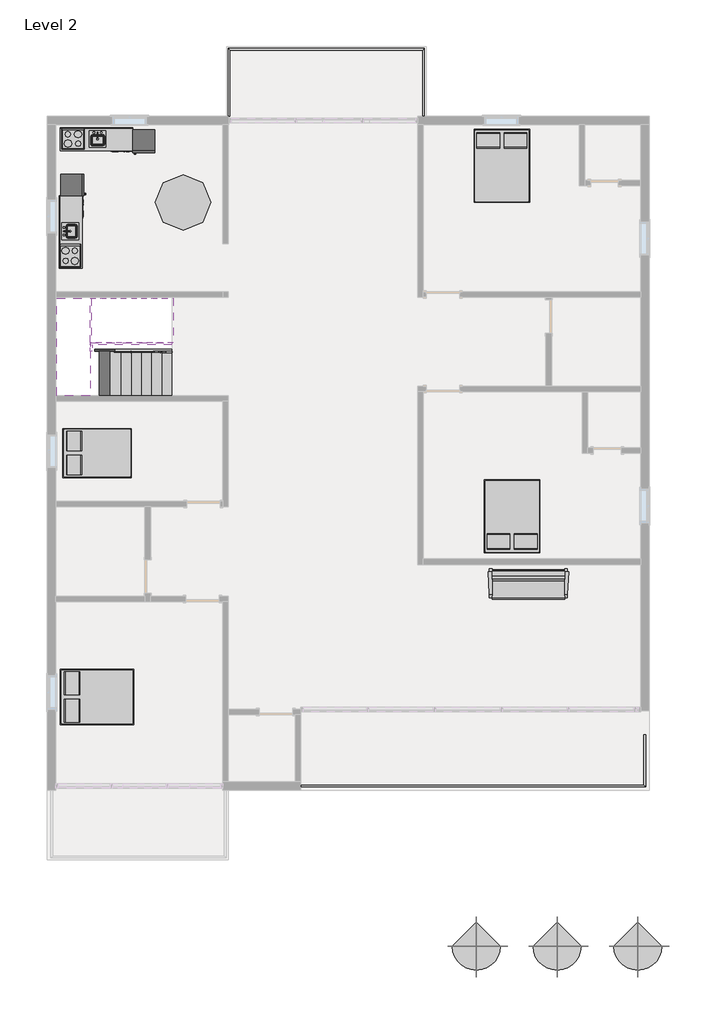
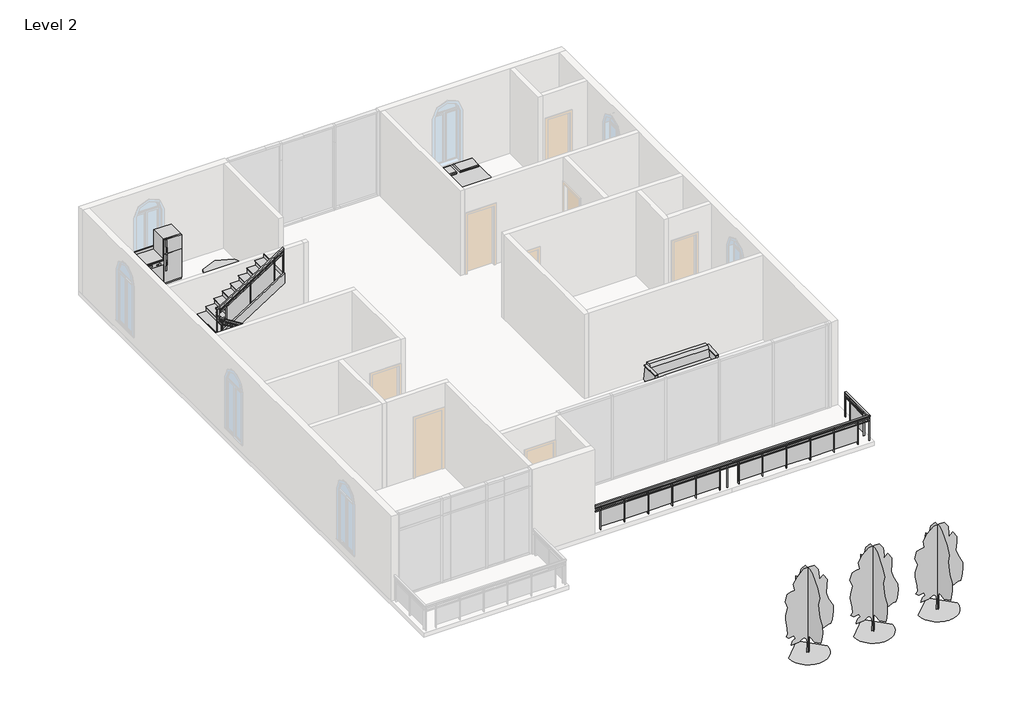
# One storey, part 3 of 3: 8 furniture elements, 8 proxies, 3 geographic elements, 3 members, 3 railings, 2 flow terminals, 2 stair flights, 1 slab.
"""IFC4 building model written with IfcOpenShell, lengths in millimetres."""

from ifc_helpers import new_model, si_unit, frame, origin, place, context, project, spatial, polyline, outline, extrude, faceted_brep, transform, mapped, element, save
from components import proxy_a6faaae8, proxy_45b28599, kitchenette_medium_kitchenette_medium_844211aa, proxy_c523a7b7, flow_terminal_871c2e40, furniture_c8abb964, furniture_1d2926bd, furniture_c6510c7c, furniture_aff9b2fb, furniture_bbcc68ce, rpc_tree_deciduous_red_ash_25_5dd3353f, non_monolithic_landing_6f104080, stair_flight_d31f5684, stair_flight_e2acd8df

model = new_model("IFC4")

# Units and contexts
model_context = context("Model", 3, world=origin())
ifc_project = project(units=[si_unit("LENGTHUNIT", "METRE", prefix="MILLI")], contexts=[model_context])

# Site, building, storey
site = spatial("IfcSite", under=ifc_project)
building = spatial("IfcBuilding", under=site)
storey = spatial("IfcBuildingStorey", under=building, Name="Level 2", Elevation=3200.4)

# Proxies
placement = place(None, origin())
proxy_shape = proxy_a6faaae8(model_context)
element("IfcBuildingElementProxy", 1, Name="Cook Top-4 Unit2 : 22\" x 20\"", ObjectType="Cook Top-4 Unit2 : 22\" x 20\"", at=placement, inside=storey, context=model_context, shape_type="MappedRepresentation", body=[
    mapped(proxy_shape, transform((-8593.3707895, 12037.2144188, 3200.4), x_axis=(1.0, 0.0, 0.0), y_axis=(0.0, 1.0, 0.0), z_axis=(0.0, 0.0, 1.0))),
])
element("IfcBuildingElementProxy", 2, Name="Cook Top-4 Unit2 : 22\" x 20\"", ObjectType="Cook Top-4 Unit2 : 22\" x 20\"", at=placement, inside=storey, context=model_context, shape_type="MappedRepresentation", body=[
    mapped(proxy_shape, transform((-8669.5707895, 8836.8144188, 3200.4), x_axis=(0.0, 1.0000000000000002, 0.0), y_axis=(-1.0000000000000002, 0.0, 0.0), z_axis=(0.0, 0.0, 1.0))),
])
proxy_2_shape = proxy_45b28599(model_context)
element("IfcBuildingElementProxy", 3, Name="Dishwasher : 24\" x 24\" x 34\"", ObjectType="Dishwasher : 24\" x 24\" x 34\"", at=placement, inside=storey, context=model_context, shape_type="MappedRepresentation", body=[
    mapped(proxy_2_shape, transform((-7642.188258, 11745.364854, 3200.4), x_axis=(1.0, 0.0, 0.0), y_axis=(0.0, 1.0, 0.0), z_axis=(0.0, 0.0, 1.0))),
])
element("IfcBuildingElementProxy", 4, Name="Dishwasher : 24\" x 24\" x 34\"", ObjectType="Dishwasher : 24\" x 24\" x 34\"", at=placement, inside=storey, context=model_context, shape_type="MappedRepresentation", body=[
    mapped(proxy_2_shape, transform((-8377.7212247, 9787.9969503, 3200.4), x_axis=(0.0, 1.0000000000000002, 0.0), y_axis=(-1.0000000000000002, 0.0, 0.0), z_axis=(0.0, 0.0, 1.0))),
])
kitchenette_medium_kitchenette_medium_shape = kitchenette_medium_kitchenette_medium_844211aa(model_context)
element("IfcBuildingElementProxy", 5, Name="Kitchenette - Medium : Kitchenette - Medium", ObjectType="Kitchenette - Medium : Kitchenette - Medium", at=placement, inside=storey, context=model_context, shape_type="MappedRepresentation", body=[
    mapped(kitchenette_medium_kitchenette_medium_shape, transform((-8269.2084944, 12342.0144188, 3200.4), x_axis=(1.0, 0.0, 0.0), y_axis=(0.0, 1.0, 0.0), z_axis=(0.0, 0.0, 1.0))),
])
element("IfcBuildingElementProxy", 6, Name="Kitchenette - Medium : Kitchenette - Medium", ObjectType="Kitchenette - Medium : Kitchenette - Medium", at=placement, inside=storey, context=model_context, shape_type="MappedRepresentation", body=[
    mapped(kitchenette_medium_kitchenette_medium_shape, transform((-8974.3707895, 9160.9767139, 3200.4), x_axis=(0.0, 1.0000000000000002, 0.0), y_axis=(-1.0000000000000002, 0.0, 0.0), z_axis=(0.0, 0.0, 1.0))),
])
proxy_3_shape = proxy_c523a7b7(model_context)
element("IfcBuildingElementProxy", 7, Name="Refrigerator : 24\" x 25\" LH", ObjectType="Refrigerator : 24\" x 25\" LH", at=placement, inside=storey, context=model_context, shape_type="MappedRepresentation", body=[
    mapped(proxy_3_shape, transform((-6656.6207895, 11991.5654473, 3200.4), x_axis=(1.0, 0.0, 0.0), y_axis=(0.0, 1.0, 0.0), z_axis=(0.0, 0.0, 1.0))),
])
element("IfcBuildingElementProxy", 8, Name="Refrigerator : 24\" x 25\" LH", ObjectType="Refrigerator : 24\" x 25\" LH", at=placement, inside=storey, context=model_context, shape_type="MappedRepresentation", body=[
    mapped(proxy_3_shape, transform((-8623.921818, 10773.5644188, 3200.4), x_axis=(0.0, 1.0000000000000002, 0.0), y_axis=(-1.0000000000000002, 0.0, 0.0), z_axis=(0.0, 0.0, 1.0))),
])

# Flow terminals
flow_terminal_shape = flow_terminal_871c2e40(model_context)
element("IfcFlowTerminal", 9, ObjectType="Sink Kitchen-Island : 18\" x 18\"", at=placement, inside=storey, context=model_context, shape_type="MappedRepresentation", body=[
    mapped(flow_terminal_shape, transform((-7935.96003, 12034.8690177, 3186.0), x_axis=(1.0, 0.0, 0.0), y_axis=(0.0, 1.0, 0.0), z_axis=(0.0, 0.0, 1.0))),
])
element("IfcFlowTerminal", 10, ObjectType="Sink Kitchen-Island : 18\" x 18\"", at=placement, inside=storey, context=model_context, shape_type="MappedRepresentation", body=[
    mapped(flow_terminal_shape, transform((-8667.2253884, 9494.2251782, 3186.0), x_axis=(0.0, 1.0000000000000002, 0.0), y_axis=(-1.0000000000000002, 0.0, 0.0), z_axis=(0.0, 0.0, 1.0))),
])

# Furniture
furniture_shape = furniture_c8abb964(model_context)
element("IfcFurniture", 11, ObjectType="Bed-Box : Double 53\" x 74\"", at=placement, inside=storey, context=model_context, shape_type="MappedRepresentation", body=[
    mapped(furniture_shape, transform((-8167.4002977, 3100.1619598, 3200.4), x_axis=(0.0, 1.0, 0.0), y_axis=(-1.0, 0.0, 0.0), z_axis=(0.0, 0.0, 1.0))),
])
furniture_2_shape = furniture_1d2926bd(model_context)
element("IfcFurniture", 12, ObjectType="Bed-Box : Queen 60\" x 79\"", at=placement, inside=storey, context=model_context, shape_type="MappedRepresentation", body=[
    mapped(furniture_2_shape, transform((-8167.4002977, -3571.0855812, 3200.4), x_axis=(0.0, 1.0000000000000002, 0.0), y_axis=(-1.0000000000000002, 0.0, 0.0), z_axis=(0.0, 0.0, 1.0))),
])
element("IfcFurniture", 13, ObjectType="Bed-Box : Queen 60\" x 79\"", at=placement, inside=storey, context=model_context, shape_type="MappedRepresentation", body=[
    mapped(furniture_2_shape, transform((3759.9816695, 1477.6849106, 3200.4), x_axis=(-1.0, 0.0, 0.0), y_axis=(0.0, -1.0, 0.0), z_axis=(0.0, 0.0, 1.0))),
])
element("IfcFurniture", 14, ObjectType="Bed-Box : Queen 60\" x 79\"", at=placement, inside=storey, context=model_context, shape_type="MappedRepresentation", body=[
    mapped(furniture_2_shape, transform((2802.2767515, 11535.043927, 3200.4), x_axis=(1.0000000000000002, 0.0, 0.0), y_axis=(0.0, 1.0000000000000002, 0.0), z_axis=(0.0, 0.0, 1.0))),
])
furniture_3_shape = furniture_c6510c7c(model_context)
element("IfcFurniture", 15, ObjectType="Counter Top w Sink Hole : 24\" Depth", at=placement, inside=storey, context=model_context, shape_type="MappedRepresentation", body=[
    mapped(furniture_3_shape, transform((-7735.8084944, 12342.0144188, 3186.0), x_axis=(1.0, 0.0, 0.0), y_axis=(0.0, 1.0, 0.0), z_axis=(0.0, 0.0, 1.0))),
])
element("IfcFurniture", 16, ObjectType="Counter Top w Sink Hole : 24\" Depth", at=placement, inside=storey, context=model_context, shape_type="MappedRepresentation", body=[
    mapped(furniture_3_shape, transform((-8974.3707895, 9694.3767139, 3186.0), x_axis=(0.0, 1.0000000000000002, 0.0), y_axis=(-1.0000000000000002, 0.0, 0.0), z_axis=(0.0, 0.0, 1.0))),
])
furniture_4_shape = furniture_aff9b2fb(model_context)
element("IfcFurniture", 17, ObjectType="Sofa-Pensi : 84\"", at=placement, inside=storey, context=model_context, shape_type="MappedRepresentation", body=[
    mapped(furniture_4_shape, transform((3586.7229605, -419.1954173, 3200.4), x_axis=(1.0, 0.0, 0.0), y_axis=(0.0, 1.0, 0.0), z_axis=(0.0, 0.0, 1.0))),
])
furniture_5_shape = furniture_bbcc68ce(model_context)
element("IfcFurniture", 18, ObjectType="Table-Dining Round w Chairs : 36\" Diameter", at=placement, inside=storey, context=model_context, shape_type="MappedRepresentation", body=[
    mapped(furniture_5_shape, transform((-5687.1527567, 10482.1931073, 3200.4), x_axis=(1.0, 0.0, 0.0), y_axis=(0.0, 1.0, 0.0), z_axis=(0.0, 0.0, 1.0))),
])

# Geographic elements
rpc_tree_deciduous_red_ash_25_shape = rpc_tree_deciduous_red_ash_25_5dd3353f(model_context)
element("IfcGeographicElement", 19, ObjectType="RPC Tree - Deciduous : Red Ash - 25'", at=placement, inside=storey, context=model_context, shape_type="MappedRepresentation", body=[
    mapped(rpc_tree_deciduous_red_ash_25_shape, transform((6861.9208729, -10048.0855812, -152.4), x_axis=(1.0, 0.0, 0.0), y_axis=(0.0, 1.0, 0.0), z_axis=(0.0, 0.0, 1.0))),
])
element("IfcGeographicElement", 20, ObjectType="RPC Tree - Deciduous : Red Ash - 25'", at=placement, inside=storey, context=model_context, shape_type="MappedRepresentation", body=[
    mapped(rpc_tree_deciduous_red_ash_25_shape, transform((4652.1208729, -10048.0855812, -152.4), x_axis=(1.0, 0.0, 0.0), y_axis=(0.0, 1.0, 0.0), z_axis=(0.0, 0.0, 1.0))),
])
element("IfcGeographicElement", 21, ObjectType="RPC Tree - Deciduous : Red Ash - 25'", at=placement, inside=storey, context=model_context, shape_type="MappedRepresentation", body=[
    mapped(rpc_tree_deciduous_red_ash_25_shape, transform((2442.3208729, -10048.0855812, -152.4), x_axis=(1.0, 0.0, 0.0), y_axis=(0.0, 1.0, 0.0), z_axis=(0.0, 0.0, 1.0))),
])

# Members
element("IfcMember", 22, ObjectType="Stringer - 2\" Width", at=placement, inside=storey, context=model_context, shape_type="SweptSolid", body=[
    extrude(outline(polyline([(3200.4, -5888.2707895), (3415.4106437, -5888.2707895), (4805.483371, -8072.6707895), (4444.2010268, -8072.6707895), (3200.4, -6118.1263188), (3200.4, -5888.2707895)])), frame((0.0, 6233.3144188, 0.0), z_axis=(0.0, 1.0, 0.0), x_axis=(0.0, 0.0, 1.0)), (0.0, 0.0, 1.0), 50.8),
])
element("IfcMember", 23, ObjectType="Stringer - 2\" Width", at=placement, inside=storey, context=model_context, shape_type="SweptSolid", body=[
    extrude(outline(polyline([(5015.6106437, -8123.4707895), (4654.3282995, -8123.4707895), (6076.7282995, -5888.2707895), (6438.0106437, -5888.2707895), (5015.6106437, -8123.4707895)])), frame((0.0, 6411.1144188, 0.0), z_axis=(0.0, 1.0, 0.0), x_axis=(0.0, 0.0, 1.0)), (0.0, 0.0, 1.0), 50.8),
])
element("IfcMember", 24, ObjectType="Stringer - 2\" Width", at=placement, inside=storey, context=model_context, shape_type="SweptSolid", body=[
    extrude(outline(polyline([(-8072.6707895, 6233.3144188), (-8123.4707895, 6233.3144188), (-8123.4707895, 6411.1144188), (-8072.6707895, 6411.1144188), (-8072.6707895, 6233.3144188)])), frame((0.0, 0.0, 4572.0), z_axis=(0.0, 0.0, 1.0), x_axis=(1.0, 0.0, 0.0)), (0.0, 0.0, 1.0), 304.8),
])

# Railings
element("IfcRailing", 25, ObjectType="Glass Panel - Bottom Fill", at=placement, inside=storey, context=model_context, shape_type="SolidModel", body=[
    faceted_brep([(-5888.2707895, 6182.5144188, 4292.6), (-5888.2707895, 6182.5144188, 4232.386276), (-5888.2707895, 6233.3144188, 4232.386276), (-5888.2707895, 6233.3144188, 4292.6), (-8047.2707895, 6182.5144188, 5666.5090909), (-8098.0707895, 6182.5144188, 5638.6226396), (-8098.0707895, 6233.3144188, 5638.6226396), (-8047.2707895, 6233.3144188, 5666.5090909), (-8174.2707895, 6309.5144188, 5664.2), (-8174.2707895, 6309.5144188, 5715.0), (-8174.2707895, 6385.7144188, 5715.0), (-8174.2707895, 6436.5144188, 5664.2), (-8123.4707895, 6309.5144188, 5664.2), (-8123.4707895, 6436.5144188, 5664.2), (-8123.4707895, 6309.5144188, 5715.0), (-8123.4707895, 6385.7144188, 5715.0), (-8174.2707895, 6385.7144188, 5941.2909091), (-8174.2707895, 6436.5144188, 5890.4909091), (-8123.4707895, 6436.5144188, 5890.4909091), (-8123.4707895, 6385.7144188, 5941.2909091), (-5888.2707895, 6512.7144188, 7315.2), (-5888.2707895, 6461.9144188, 7315.2), (-5888.2707895, 6461.9144188, 7254.986276), (-5888.2707895, 6512.7144188, 7254.986276), (-8032.4777946, 6512.7144188, 5890.4909091), (-8047.2707895, 6512.7144188, 5941.2909091), (-8032.4777946, 6461.9144188, 5890.4909091), (-8047.2707895, 6461.9144188, 5941.2909091), (-8047.2707895, 6182.5144188, 5715.0), (-8098.0707895, 6182.5144188, 5664.2), (-8098.0707895, 6233.3144188, 5664.2), (-8047.2707895, 6233.3144188, 5715.0), (-8174.2707895, 6182.5144188, 5715.0), (-8174.2707895, 6182.5144188, 5664.2), (-8123.4707895, 6233.3144188, 5664.2), (-8123.4707895, 6233.3144188, 5715.0), (-8174.2707895, 6512.7144188, 5941.2909091), (-8174.2707895, 6512.7144188, 5890.4909091), (-8123.4707895, 6461.9144188, 5890.4909091), (-8123.4707895, 6461.9144188, 5941.2909091)], [[[0, 1, 2, 3]], [[1, 0, 4, 5]], [[2, 1, 5, 6]], [[3, 2, 6, 7]], [[0, 3, 7, 4]], [[8, 9, 10, 11]], [[12, 8, 11, 13]], [[14, 12, 13, 15]], [[9, 14, 15, 10]], [[11, 10, 16, 17]], [[13, 11, 17, 18]], [[15, 13, 18, 19]], [[10, 15, 19, 16]], [[20, 21, 22, 23]], [[24, 25, 20, 23]], [[26, 24, 23, 22]], [[27, 26, 22, 21]], [[25, 27, 21, 20]], [[5, 4, 28, 29]], [[6, 5, 29, 30]], [[7, 6, 30, 31]], [[4, 7, 31, 28]], [[29, 28, 32, 33]], [[30, 29, 33, 34]], [[31, 30, 34, 35]], [[28, 31, 35, 32]], [[33, 32, 9, 8]], [[34, 33, 8, 12]], [[35, 34, 12, 14]], [[32, 35, 14, 9]], [[17, 16, 36, 37]], [[18, 17, 37, 38]], [[19, 18, 38, 39]], [[16, 19, 39, 36]], [[37, 36, 25, 24]], [[38, 37, 24, 26]], [[39, 38, 26, 27]], [[36, 39, 27, 25]]]),
    faceted_brep([(-5888.2707895, 6220.6144188, 4206.053431), (-5888.2707895, 6195.2144188, 4206.053431), (-5888.2707895, 6195.2144188, 4175.946569), (-5888.2707895, 6220.6144188, 4175.946569), (-8119.7725408, 6220.6144188, 5626.1), (-8119.7725408, 6195.2144188, 5626.1), (-8127.1690382, 6195.2144188, 5600.7), (-8127.1690382, 6220.6144188, 5600.7), (-8136.1707895, 6220.6144188, 5626.1), (-8161.5707895, 6195.2144188, 5626.1), (-8161.5707895, 6195.2144188, 5600.7), (-8136.1707895, 6220.6144188, 5600.7), (-8136.1707895, 6474.6144188, 5626.1), (-8136.1707895, 6474.6144188, 5600.7), (-8161.5707895, 6474.6144188, 5600.7), (-8161.5707895, 6474.6144188, 5626.1)], [[[0, 1, 2, 3]], [[1, 0, 4, 5]], [[2, 1, 5, 6]], [[3, 2, 6, 7]], [[0, 3, 7, 4]], [[5, 4, 8, 9]], [[6, 5, 9, 10]], [[7, 6, 10, 11]], [[4, 7, 11, 8]], [[12, 13, 14, 15]], [[9, 8, 12, 15]], [[10, 9, 15, 14]], [[11, 10, 14, 13]], [[8, 11, 13, 12]]]),
    faceted_brep([(-8161.5707895, 6474.6144188, 5782.0079765), (-8161.5707895, 6500.0144188, 5782.0079765), (-8161.5707895, 6500.0144188, 5751.9011144), (-8161.5707895, 6474.6144188, 5751.9011144), (-5888.2707895, 6474.6144188, 7228.653431), (-5888.2707895, 6474.6144188, 7198.546569), (-5888.2707895, 6500.0144188, 7198.546569), (-5888.2707895, 6500.0144188, 7228.653431)], [[[0, 1, 2, 3]], [[4, 5, 6, 7]], [[1, 0, 4, 7]], [[2, 1, 7, 6]], [[3, 2, 6, 5]], [[0, 3, 5, 4]]]),
    faceted_brep([(-5888.2707895, 6220.6144188, 4104.453431), (-5888.2707895, 6195.2144188, 4104.453431), (-5888.2707895, 6195.2144188, 4074.346569), (-5888.2707895, 6220.6144188, 4074.346569), (-8119.7725408, 6220.6144188, 5524.5), (-8119.7725408, 6195.2144188, 5524.5), (-8127.1690382, 6195.2144188, 5499.1), (-8127.1690382, 6220.6144188, 5499.1), (-8136.1707895, 6220.6144188, 5524.5), (-8161.5707895, 6195.2144188, 5524.5), (-8161.5707895, 6195.2144188, 5499.1), (-8136.1707895, 6220.6144188, 5499.1), (-8136.1707895, 6474.6144188, 5524.5), (-8136.1707895, 6474.6144188, 5499.1), (-8161.5707895, 6474.6144188, 5499.1), (-8161.5707895, 6474.6144188, 5524.5)], [[[0, 1, 2, 3]], [[1, 0, 4, 5]], [[2, 1, 5, 6]], [[3, 2, 6, 7]], [[0, 3, 7, 4]], [[5, 4, 8, 9]], [[6, 5, 9, 10]], [[7, 6, 10, 11]], [[4, 7, 11, 8]], [[12, 13, 14, 15]], [[9, 8, 12, 15]], [[10, 9, 15, 14]], [[11, 10, 14, 13]], [[8, 11, 13, 12]]]),
    faceted_brep([(-8161.5707895, 6474.6144188, 5680.4079765), (-8161.5707895, 6500.0144188, 5680.4079765), (-8161.5707895, 6500.0144188, 5650.3011144), (-8161.5707895, 6474.6144188, 5650.3011144), (-5888.2707895, 6474.6144188, 7127.053431), (-5888.2707895, 6474.6144188, 7096.946569), (-5888.2707895, 6500.0144188, 7096.946569), (-5888.2707895, 6500.0144188, 7127.053431)], [[[0, 1, 2, 3]], [[4, 5, 6, 7]], [[1, 0, 4, 7]], [[2, 1, 7, 6]], [[3, 2, 6, 5]], [[0, 3, 5, 4]]]),
    extrude(outline(polyline([(7056.9817305, -6199.4207895), (7048.8999123, -6212.1207895), (6045.2, -6212.1207895), (6045.2, -6199.4207895), (7056.9817305, -6199.4207895)])), frame((0.0, 6461.9144188, 0.0), z_axis=(0.0, 1.0, 0.0), x_axis=(0.0, 0.0, 1.0)), (0.0, 0.0, 1.0), 50.8),
    extrude(outline(polyline([(5710.3818182, -7018.5707895), (6227.6181818, -6205.7707895), (6894.9011144, -6205.7707895), (6377.6647508, -7018.5707895), (5710.3818182, -7018.5707895)])), frame((0.0, 6487.4995758, 0.0), z_axis=(0.0, 1.0, 0.0), x_axis=(0.0, 0.0, 1.0)), (0.0, 0.0, 1.0), 6.35),
    extrude(outline(polyline([(6539.7453669, -7012.2207895), (6531.6635487, -7024.9207895), (5511.8, -7024.9207895), (5511.8, -7012.2207895), (6539.7453669, -7012.2207895)])), frame((0.0, 6461.9144188, 0.0), z_axis=(0.0, 1.0, 0.0), x_axis=(0.0, 0.0, 1.0)), (0.0, 0.0, 1.0), 50.8),
    extrude(outline(polyline([(5176.9818182, -7831.3707895), (5694.2181818, -7018.5707895), (6377.6647508, -7018.5707895), (5860.4283872, -7831.3707895), (5176.9818182, -7831.3707895)])), frame((0.0, 6487.4995758, 0.0), z_axis=(0.0, 1.0, 0.0), x_axis=(0.0, 0.0, 1.0)), (0.0, 0.0, 1.0), 6.35),
    extrude(outline(polyline([(6022.5090032, -7825.0207895), (6014.4271851, -7837.7207895), (5156.2, -7837.7207895), (5156.2, -7825.0207895), (6022.5090032, -7825.0207895)])), frame((0.0, 6461.9144188, 0.0), z_axis=(0.0, 1.0, 0.0), x_axis=(0.0, 0.0, 1.0)), (0.0, 0.0, 1.0), 50.8),
    extrude(outline(polyline([(5456.7817305, -7812.3207895), (5464.8635487, -7825.0207895), (4445.0, -7825.0207895), (4445.0, -7812.3207895), (5456.7817305, -7812.3207895)])), frame((0.0, 6182.5144188, 0.0), z_axis=(0.0, 1.0, 0.0), x_axis=(0.0, 0.0, 1.0)), (0.0, 0.0, 1.0), 50.8),
    extrude(outline(polyline([(4110.1818182, -7005.8707895), (4785.546569, -7005.8707895), (5302.7829326, -7818.6707895), (4627.4181818, -7818.6707895), (4110.1818182, -7005.8707895)])), frame((0.0, 6201.3792618, 0.0), z_axis=(0.0, 1.0, 0.0), x_axis=(0.0, 0.0, 1.0)), (0.0, 0.0, 1.0), 6.35),
    extrude(outline(polyline([(4939.5453669, -6999.5207895), (4947.6271851, -7012.2207895), (4089.4, -7012.2207895), (4089.4, -6999.5207895), (4939.5453669, -6999.5207895)])), frame((0.0, 6182.5144188, 0.0), z_axis=(0.0, 1.0, 0.0), x_axis=(0.0, 0.0, 1.0)), (0.0, 0.0, 1.0), 50.8),
    extrude(outline(polyline([(3576.7818182, -6193.0707895), (4268.3102054, -6193.0707895), (4785.546569, -7005.8707895), (4094.0181818, -7005.8707895), (3576.7818182, -6193.0707895)])), frame((0.0, 6201.3792618, 0.0), z_axis=(0.0, 1.0, 0.0), x_axis=(0.0, 0.0, 1.0)), (0.0, 0.0, 1.0), 6.35),
    extrude(outline(polyline([(4422.3090032, -6186.7207895), (4430.3908214, -6199.4207895), (3556.0, -6199.4207895), (3556.0, -6186.7207895), (4422.3090032, -6186.7207895)])), frame((0.0, 6182.5144188, 0.0), z_axis=(0.0, 1.0, 0.0), x_axis=(0.0, 0.0, 1.0)), (0.0, 0.0, 1.0), 50.8),
    extrude(outline(polyline([(-8158.3957895, 6477.7894188), (-8158.3957895, 6496.8394188), (-8139.3457895, 6496.8394188), (-8139.3457895, 6477.7894188), (-8158.3957895, 6477.7894188)])), frame((0.0, 0.0, 4800.6), z_axis=(0.0, 0.0, 1.0), x_axis=(1.0, 0.0, 0.0)), (0.0, 0.0, 1.0), 1089.8909091),
    extrude(outline(polyline([(-8139.3457895, 6217.4394188), (-8139.3457895, 6198.3894188), (-8158.3957895, 6198.3894188), (-8158.3957895, 6217.4394188), (-8139.3457895, 6217.4394188)])), frame((0.0, 0.0, 4800.6), z_axis=(0.0, 0.0, 1.0), x_axis=(1.0, 0.0, 0.0)), (0.0, 0.0, 1.0), 863.6),
    extrude(outline(polyline([(-8113.9457895, 6217.4394188), (-8113.9457895, 6198.3894188), (-8132.9957895, 6198.3894188), (-8132.9957895, 6217.4394188), (-8113.9457895, 6217.4394188)])), frame((0.0, 0.0, 4800.6), z_axis=(0.0, 0.0, 1.0), x_axis=(1.0, 0.0, 0.0)), (0.0, 0.0, 1.0), 863.6),
    extrude(outline(polyline([(7259.0271851, -5881.9207895), (7246.9044578, -5900.9707895), (6223.0, -5900.9707895), (6223.0, -5881.9207895), (7259.0271851, -5881.9207895)])), frame((0.0, 6477.7894188, 0.0), z_axis=(0.0, 1.0, 0.0), x_axis=(0.0, 0.0, 1.0)), (0.0, 0.0, 1.0), 19.05),
    extrude(outline(polyline([(4228.3453669, -5881.9207895), (4240.4680941, -5900.9707895), (3378.2, -5900.9707895), (3378.2, -5881.9207895), (4228.3453669, -5881.9207895)])), frame((0.0, 6198.3894188, 0.0), z_axis=(0.0, 1.0, 0.0), x_axis=(0.0, 0.0, 1.0)), (0.0, 0.0, 1.0), 19.05),
])
element("IfcRailing", 26, ObjectType="Glass Panel - Bottom Fill", at=placement, inside=storey, context=model_context, shape_type="SolidModel", body=[
    faceted_brep([(-2357.6707895, -5641.1855812, 4114.8), (-2357.6707895, -5641.1855812, 4064.0), (-2357.6707895, -5691.9855812, 4064.0), (-2357.6707895, -5691.9855812, 4114.8), (7027.6292105, -5641.1855812, 4114.8), (7027.6292105, -5641.1855812, 4064.0), (7078.4292105, -5691.9855812, 4064.0), (7078.4292105, -5691.9855812, 4114.8), (7027.6292105, -4266.4105812, 4114.8), (7078.4292105, -4266.4105812, 4114.8), (7078.4292105, -4266.4105812, 4064.0), (7027.6292105, -4266.4105812, 4064.0)], [[[0, 1, 2, 3]], [[1, 0, 4, 5]], [[2, 1, 5, 6]], [[3, 2, 6, 7]], [[0, 3, 7, 4]], [[8, 9, 10, 11]], [[5, 4, 8, 11]], [[6, 5, 11, 10]], [[7, 6, 10, 9]], [[4, 7, 9, 8]]]),
    faceted_brep([(-2357.6707895, -5679.2855812, 4025.9), (-2357.6707895, -5653.8855812, 4025.9), (-2357.6707895, -5653.8855812, 4000.5), (-2357.6707895, -5679.2855812, 4000.5), (7065.7292105, -5679.2855812, 4025.9), (7040.3292105, -5653.8855812, 4025.9), (7040.3292105, -5653.8855812, 4000.5), (7065.7292105, -5679.2855812, 4000.5), (7065.7292105, -4266.4105812, 4025.9), (7065.7292105, -4266.4105812, 4000.5), (7040.3292105, -4266.4105812, 4000.5), (7040.3292105, -4266.4105812, 4025.9)], [[[0, 1, 2, 3]], [[1, 0, 4, 5]], [[2, 1, 5, 6]], [[3, 2, 6, 7]], [[0, 3, 7, 4]], [[8, 9, 10, 11]], [[5, 4, 8, 11]], [[6, 5, 11, 10]], [[7, 6, 10, 9]], [[4, 7, 9, 8]]]),
    faceted_brep([(-2357.6707895, -5679.2855812, 3924.3), (-2357.6707895, -5653.8855812, 3924.3), (-2357.6707895, -5653.8855812, 3898.9), (-2357.6707895, -5679.2855812, 3898.9), (7065.7292105, -5679.2855812, 3924.3), (7040.3292105, -5653.8855812, 3924.3), (7040.3292105, -5653.8855812, 3898.9), (7065.7292105, -5679.2855812, 3898.9), (7065.7292105, -4266.4105812, 3924.3), (7065.7292105, -4266.4105812, 3898.9), (7040.3292105, -4266.4105812, 3898.9), (7040.3292105, -4266.4105812, 3924.3)], [[[0, 1, 2, 3]], [[1, 0, 4, 5]], [[2, 1, 5, 6]], [[3, 2, 6, 7]], [[0, 3, 7, 4]], [[8, 9, 10, 11]], [[5, 4, 8, 11]], [[6, 5, 11, 10]], [[7, 6, 10, 9]], [[4, 7, 9, 8]]]),
    extrude(outline(polyline([(7078.4292105, -4566.4480812), (7027.6292105, -4566.4480812), (7027.6292105, -4553.7480812), (7078.4292105, -4553.7480812), (7078.4292105, -4566.4480812)])), frame((0.0, 0.0, 3200.4), z_axis=(0.0, 0.0, 1.0), x_axis=(1.0, 0.0, 0.0)), (0.0, 0.0, 1.0), 863.6),
    extrude(outline(polyline([(7046.4940535, -5372.8980812), (7046.4940535, -4560.0980812), (7052.8440535, -4560.0980812), (7052.8440535, -5372.8980812), (7046.4940535, -5372.8980812)])), frame((0.0, 0.0, 3302.0), z_axis=(0.0, 0.0, 1.0), x_axis=(1.0, 0.0, 0.0)), (0.0, 0.0, 1.0), 596.9),
    extrude(outline(polyline([(7078.4292105, -5379.2480812), (7027.6292105, -5379.2480812), (7027.6292105, -5366.5480812), (7078.4292105, -5366.5480812), (7078.4292105, -5379.2480812)])), frame((0.0, 0.0, 3200.4), z_axis=(0.0, 0.0, 1.0), x_axis=(1.0, 0.0, 0.0)), (0.0, 0.0, 1.0), 863.6),
    extrude(outline(polyline([(6659.3292105, -5691.9855812), (6659.3292105, -5641.1855812), (6672.0292105, -5641.1855812), (6672.0292105, -5691.9855812), (6659.3292105, -5691.9855812)])), frame((0.0, 0.0, 3200.4), z_axis=(0.0, 0.0, 1.0), x_axis=(1.0, 0.0, 0.0)), (0.0, 0.0, 1.0), 863.6),
    extrude(outline(polyline([(5852.8792105, -5660.0504242), (6665.6792105, -5660.0504242), (6665.6792105, -5666.4004242), (5852.8792105, -5666.4004242), (5852.8792105, -5660.0504242)])), frame((0.0, 0.0, 3302.0), z_axis=(0.0, 0.0, 1.0), x_axis=(1.0, 0.0, 0.0)), (0.0, 0.0, 1.0), 596.9),
    extrude(outline(polyline([(5846.5292105, -5691.9855812), (5846.5292105, -5641.1855812), (5859.2292105, -5641.1855812), (5859.2292105, -5691.9855812), (5846.5292105, -5691.9855812)])), frame((0.0, 0.0, 3200.4), z_axis=(0.0, 0.0, 1.0), x_axis=(1.0, 0.0, 0.0)), (0.0, 0.0, 1.0), 863.6),
    extrude(outline(polyline([(5040.0792105, -5660.0504242), (5852.8792105, -5660.0504242), (5852.8792105, -5666.4004242), (5040.0792105, -5666.4004242), (5040.0792105, -5660.0504242)])), frame((0.0, 0.0, 3302.0), z_axis=(0.0, 0.0, 1.0), x_axis=(1.0, 0.0, 0.0)), (0.0, 0.0, 1.0), 596.9),
    extrude(outline(polyline([(5033.7292105, -5691.9855812), (5033.7292105, -5641.1855812), (5046.4292105, -5641.1855812), (5046.4292105, -5691.9855812), (5033.7292105, -5691.9855812)])), frame((0.0, 0.0, 3200.4), z_axis=(0.0, 0.0, 1.0), x_axis=(1.0, 0.0, 0.0)), (0.0, 0.0, 1.0), 863.6),
    extrude(outline(polyline([(4227.2792105, -5660.0504242), (5040.0792105, -5660.0504242), (5040.0792105, -5666.4004242), (4227.2792105, -5666.4004242), (4227.2792105, -5660.0504242)])), frame((0.0, 0.0, 3302.0), z_axis=(0.0, 0.0, 1.0), x_axis=(1.0, 0.0, 0.0)), (0.0, 0.0, 1.0), 596.9),
    extrude(outline(polyline([(4220.9292105, -5691.9855812), (4220.9292105, -5641.1855812), (4233.6292105, -5641.1855812), (4233.6292105, -5691.9855812), (4220.9292105, -5691.9855812)])), frame((0.0, 0.0, 3200.4), z_axis=(0.0, 0.0, 1.0), x_axis=(1.0, 0.0, 0.0)), (0.0, 0.0, 1.0), 863.6),
    extrude(outline(polyline([(3414.4792105, -5660.0504242), (4227.2792105, -5660.0504242), (4227.2792105, -5666.4004242), (3414.4792105, -5666.4004242), (3414.4792105, -5660.0504242)])), frame((0.0, 0.0, 3302.0), z_axis=(0.0, 0.0, 1.0), x_axis=(1.0, 0.0, 0.0)), (0.0, 0.0, 1.0), 596.9),
    extrude(outline(polyline([(3408.1292105, -5691.9855812), (3408.1292105, -5641.1855812), (3420.8292105, -5641.1855812), (3420.8292105, -5691.9855812), (3408.1292105, -5691.9855812)])), frame((0.0, 0.0, 3200.4), z_axis=(0.0, 0.0, 1.0), x_axis=(1.0, 0.0, 0.0)), (0.0, 0.0, 1.0), 863.6),
    extrude(outline(polyline([(2601.6792105, -5660.0504242), (3414.4792105, -5660.0504242), (3414.4792105, -5666.4004242), (2601.6792105, -5666.4004242), (2601.6792105, -5660.0504242)])), frame((0.0, 0.0, 3302.0), z_axis=(0.0, 0.0, 1.0), x_axis=(1.0, 0.0, 0.0)), (0.0, 0.0, 1.0), 596.9),
    extrude(outline(polyline([(2595.3292105, -5691.9855812), (2595.3292105, -5641.1855812), (2608.0292105, -5641.1855812), (2608.0292105, -5691.9855812), (2595.3292105, -5691.9855812)])), frame((0.0, 0.0, 3200.4), z_axis=(0.0, 0.0, 1.0), x_axis=(1.0, 0.0, 0.0)), (0.0, 0.0, 1.0), 863.6),
    extrude(outline(polyline([(1953.9792105, -5691.9855812), (1953.9792105, -5641.1855812), (1966.6792105, -5641.1855812), (1966.6792105, -5691.9855812), (1953.9792105, -5691.9855812)])), frame((0.0, 0.0, 3200.4), z_axis=(0.0, 0.0, 1.0), x_axis=(1.0, 0.0, 0.0)), (0.0, 0.0, 1.0), 863.6),
    extrude(outline(polyline([(1147.5292105, -5660.0504242), (1960.3292105, -5660.0504242), (1960.3292105, -5666.4004242), (1147.5292105, -5666.4004242), (1147.5292105, -5660.0504242)])), frame((0.0, 0.0, 3302.0), z_axis=(0.0, 0.0, 1.0), x_axis=(1.0, 0.0, 0.0)), (0.0, 0.0, 1.0), 596.9),
    extrude(outline(polyline([(1141.1792105, -5691.9855812), (1141.1792105, -5641.1855812), (1153.8792105, -5641.1855812), (1153.8792105, -5691.9855812), (1141.1792105, -5691.9855812)])), frame((0.0, 0.0, 3200.4), z_axis=(0.0, 0.0, 1.0), x_axis=(1.0, 0.0, 0.0)), (0.0, 0.0, 1.0), 863.6),
    extrude(outline(polyline([(334.7292105, -5660.0504242), (1147.5292105, -5660.0504242), (1147.5292105, -5666.4004242), (334.7292105, -5666.4004242), (334.7292105, -5660.0504242)])), frame((0.0, 0.0, 3302.0), z_axis=(0.0, 0.0, 1.0), x_axis=(1.0, 0.0, 0.0)), (0.0, 0.0, 1.0), 596.9),
    extrude(outline(polyline([(328.3792105, -5691.9855812), (328.3792105, -5641.1855812), (341.0792105, -5641.1855812), (341.0792105, -5691.9855812), (328.3792105, -5691.9855812)])), frame((0.0, 0.0, 3200.4), z_axis=(0.0, 0.0, 1.0), x_axis=(1.0, 0.0, 0.0)), (0.0, 0.0, 1.0), 863.6),
    extrude(outline(polyline([(-478.0707895, -5660.0504242), (334.7292105, -5660.0504242), (334.7292105, -5666.4004242), (-478.0707895, -5666.4004242), (-478.0707895, -5660.0504242)])), frame((0.0, 0.0, 3302.0), z_axis=(0.0, 0.0, 1.0), x_axis=(1.0, 0.0, 0.0)), (0.0, 0.0, 1.0), 596.9),
    extrude(outline(polyline([(-484.4207895, -5691.9855812), (-484.4207895, -5641.1855812), (-471.7207895, -5641.1855812), (-471.7207895, -5691.9855812), (-484.4207895, -5691.9855812)])), frame((0.0, 0.0, 3200.4), z_axis=(0.0, 0.0, 1.0), x_axis=(1.0, 0.0, 0.0)), (0.0, 0.0, 1.0), 863.6),
    extrude(outline(polyline([(-1290.8707895, -5660.0504242), (-478.0707895, -5660.0504242), (-478.0707895, -5666.4004242), (-1290.8707895, -5666.4004242), (-1290.8707895, -5660.0504242)])), frame((0.0, 0.0, 3302.0), z_axis=(0.0, 0.0, 1.0), x_axis=(1.0, 0.0, 0.0)), (0.0, 0.0, 1.0), 596.9),
    extrude(outline(polyline([(-1297.2207895, -5691.9855812), (-1297.2207895, -5641.1855812), (-1284.5207895, -5641.1855812), (-1284.5207895, -5691.9855812), (-1297.2207895, -5691.9855812)])), frame((0.0, 0.0, 3200.4), z_axis=(0.0, 0.0, 1.0), x_axis=(1.0, 0.0, 0.0)), (0.0, 0.0, 1.0), 863.6),
    extrude(outline(polyline([(-2103.6707895, -5660.0504242), (-1290.8707895, -5660.0504242), (-1290.8707895, -5666.4004242), (-2103.6707895, -5666.4004242), (-2103.6707895, -5660.0504242)])), frame((0.0, 0.0, 3302.0), z_axis=(0.0, 0.0, 1.0), x_axis=(1.0, 0.0, 0.0)), (0.0, 0.0, 1.0), 596.9),
    extrude(outline(polyline([(-2110.0207895, -5691.9855812), (-2110.0207895, -5641.1855812), (-2097.3207895, -5641.1855812), (-2097.3207895, -5691.9855812), (-2110.0207895, -5691.9855812)])), frame((0.0, 0.0, 3200.4), z_axis=(0.0, 0.0, 1.0), x_axis=(1.0, 0.0, 0.0)), (0.0, 0.0, 1.0), 863.6),
    extrude(outline(polyline([(7043.5042105, -5676.1105812), (7043.5042105, -5657.0605812), (7062.5542105, -5657.0605812), (7062.5542105, -5676.1105812), (7043.5042105, -5676.1105812)])), frame((0.0, 0.0, 3200.4), z_axis=(0.0, 0.0, 1.0), x_axis=(1.0, 0.0, 0.0)), (0.0, 0.0, 1.0), 863.6),
    extrude(outline(polyline([(2204.8042105, -5676.1105812), (2204.8042105, -5657.0605812), (2223.8542105, -5657.0605812), (2223.8542105, -5676.1105812), (2204.8042105, -5676.1105812)])), frame((0.0, 0.0, 3200.4), z_axis=(0.0, 0.0, 1.0), x_axis=(1.0, 0.0, 0.0)), (0.0, 0.0, 1.0), 863.6),
    extrude(outline(polyline([(7062.5542105, -4279.1105812), (7043.5042105, -4279.1105812), (7043.5042105, -4260.0605812), (7062.5542105, -4260.0605812), (7062.5542105, -4279.1105812)])), frame((0.0, 0.0, 3200.4), z_axis=(0.0, 0.0, 1.0), x_axis=(1.0, 0.0, 0.0)), (0.0, 0.0, 1.0), 863.6),
    extrude(outline(polyline([(-2364.0207895, -5676.1105812), (-2364.0207895, -5657.0605812), (-2344.9707895, -5657.0605812), (-2344.9707895, -5676.1105812), (-2364.0207895, -5676.1105812)])), frame((0.0, 0.0, 3200.4), z_axis=(0.0, 0.0, 1.0), x_axis=(1.0, 0.0, 0.0)), (0.0, 0.0, 1.0), 863.6),
])
element("IfcRailing", 27, ObjectType="Glass Panel - Bottom Fill", at=placement, inside=storey, context=model_context, shape_type="SolidModel", body=[
    faceted_brep([(-4351.5707895, 12659.5144188, 4114.8), (-4351.5707895, 12659.5144188, 4064.0), (-4300.7707895, 12659.5144188, 4064.0), (-4300.7707895, 12659.5144188, 4114.8), (-4351.5707895, 14513.7144188, 4114.8), (-4351.5707895, 14513.7144188, 4064.0), (-4300.7707895, 14462.9144188, 4064.0), (-4300.7707895, 14462.9144188, 4114.8), (1020.5292105, 14513.7144188, 4114.8), (1020.5292105, 14513.7144188, 4064.0), (969.7292105, 14462.9144188, 4064.0), (969.7292105, 14462.9144188, 4114.8), (1020.5292105, 12659.5953048, 4114.8), (969.7292105, 12659.5953048, 4114.8), (969.7292105, 12659.5953048, 4064.0), (1020.5292105, 12659.5953048, 4064.0)], [[[0, 1, 2, 3]], [[1, 0, 4, 5]], [[2, 1, 5, 6]], [[3, 2, 6, 7]], [[0, 3, 7, 4]], [[5, 4, 8, 9]], [[6, 5, 9, 10]], [[7, 6, 10, 11]], [[4, 7, 11, 8]], [[12, 13, 14, 15]], [[9, 8, 12, 15]], [[10, 9, 15, 14]], [[11, 10, 14, 13]], [[8, 11, 13, 12]]]),
    faceted_brep([(-4313.4707895, 12659.5144188, 4025.9), (-4338.8707895, 12659.5144188, 4025.9), (-4338.8707895, 12659.5144188, 4000.5), (-4313.4707895, 12659.5144188, 4000.5), (-4313.4707895, 14475.6144188, 4025.9), (-4338.8707895, 14501.0144188, 4025.9), (-4338.8707895, 14501.0144188, 4000.5), (-4313.4707895, 14475.6144188, 4000.5), (982.4292105, 14475.6144188, 4025.9), (1007.8292105, 14501.0144188, 4025.9), (1007.8292105, 14501.0144188, 4000.5), (982.4292105, 14475.6144188, 4000.5), (982.4292105, 12659.5953048, 4025.9), (982.4292105, 12659.5953048, 4000.5), (1007.8292105, 12659.5953048, 4000.5), (1007.8292105, 12659.5953048, 4025.9)], [[[0, 1, 2, 3]], [[1, 0, 4, 5]], [[2, 1, 5, 6]], [[3, 2, 6, 7]], [[0, 3, 7, 4]], [[5, 4, 8, 9]], [[6, 5, 9, 10]], [[7, 6, 10, 11]], [[4, 7, 11, 8]], [[12, 13, 14, 15]], [[9, 8, 12, 15]], [[10, 9, 15, 14]], [[11, 10, 14, 13]], [[8, 11, 13, 12]]]),
    faceted_brep([(-4313.4707895, 12659.5144188, 3924.3), (-4338.8707895, 12659.5144188, 3924.3), (-4338.8707895, 12659.5144188, 3898.9), (-4313.4707895, 12659.5144188, 3898.9), (-4313.4707895, 14475.6144188, 3924.3), (-4338.8707895, 14501.0144188, 3924.3), (-4338.8707895, 14501.0144188, 3898.9), (-4313.4707895, 14475.6144188, 3898.9), (982.4292105, 14475.6144188, 3924.3), (1007.8292105, 14501.0144188, 3924.3), (1007.8292105, 14501.0144188, 3898.9), (982.4292105, 14475.6144188, 3898.9), (982.4292105, 12659.5953048, 3924.3), (982.4292105, 12659.5953048, 3898.9), (1007.8292105, 12659.5953048, 3898.9), (1007.8292105, 12659.5953048, 3924.3)], [[[0, 1, 2, 3]], [[1, 0, 4, 5]], [[2, 1, 5, 6]], [[3, 2, 6, 7]], [[0, 3, 7, 4]], [[5, 4, 8, 9]], [[6, 5, 9, 10]], [[7, 6, 10, 11]], [[4, 7, 11, 8]], [[12, 13, 14, 15]], [[9, 8, 12, 15]], [[10, 9, 15, 14]], [[11, 10, 14, 13]], [[8, 11, 13, 12]]]),
    extrude(outline(polyline([(969.7292105, 12767.5048618), (1020.5292105, 12767.5048618), (1020.5292105, 12754.8048618), (969.7292105, 12754.8048618), (969.7292105, 12767.5048618)])), frame((0.0, 0.0, 3200.4), z_axis=(0.0, 0.0, 1.0), x_axis=(1.0, 0.0, 0.0)), (0.0, 0.0, 1.0), 863.6),
    extrude(outline(polyline([(1001.6643675, 13573.9548618), (1001.6643675, 12761.1548618), (995.3143675, 12761.1548618), (995.3143675, 13573.9548618), (1001.6643675, 13573.9548618)])), frame((0.0, 0.0, 3302.0), z_axis=(0.0, 0.0, 1.0), x_axis=(1.0, 0.0, 0.0)), (0.0, 0.0, 1.0), 596.9),
    extrude(outline(polyline([(969.7292105, 13580.3048618), (1020.5292105, 13580.3048618), (1020.5292105, 13567.6048618), (969.7292105, 13567.6048618), (969.7292105, 13580.3048618)])), frame((0.0, 0.0, 3200.4), z_axis=(0.0, 0.0, 1.0), x_axis=(1.0, 0.0, 0.0)), (0.0, 0.0, 1.0), 863.6),
    extrude(outline(polyline([(1001.6643675, 14386.7548618), (1001.6643675, 13573.9548618), (995.3143675, 13573.9548618), (995.3143675, 14386.7548618), (1001.6643675, 14386.7548618)])), frame((0.0, 0.0, 3302.0), z_axis=(0.0, 0.0, 1.0), x_axis=(1.0, 0.0, 0.0)), (0.0, 0.0, 1.0), 596.9),
    extrude(outline(polyline([(969.7292105, 14393.1048618), (1020.5292105, 14393.1048618), (1020.5292105, 14380.4048618), (969.7292105, 14380.4048618), (969.7292105, 14393.1048618)])), frame((0.0, 0.0, 3200.4), z_axis=(0.0, 0.0, 1.0), x_axis=(1.0, 0.0, 0.0)), (0.0, 0.0, 1.0), 863.6),
    extrude(outline(polyline([(766.5292105, 14462.9144188), (766.5292105, 14513.7144188), (779.2292105, 14513.7144188), (779.2292105, 14462.9144188), (766.5292105, 14462.9144188)])), frame((0.0, 0.0, 3200.4), z_axis=(0.0, 0.0, 1.0), x_axis=(1.0, 0.0, 0.0)), (0.0, 0.0, 1.0), 863.6),
    extrude(outline(polyline([(-39.9207895, 14494.8495758), (772.8792105, 14494.8495758), (772.8792105, 14488.4995758), (-39.9207895, 14488.4995758), (-39.9207895, 14494.8495758)])), frame((0.0, 0.0, 3302.0), z_axis=(0.0, 0.0, 1.0), x_axis=(1.0, 0.0, 0.0)), (0.0, 0.0, 1.0), 596.9),
    extrude(outline(polyline([(-46.2707895, 14462.9144188), (-46.2707895, 14513.7144188), (-33.5707895, 14513.7144188), (-33.5707895, 14462.9144188), (-46.2707895, 14462.9144188)])), frame((0.0, 0.0, 3200.4), z_axis=(0.0, 0.0, 1.0), x_axis=(1.0, 0.0, 0.0)), (0.0, 0.0, 1.0), 863.6),
    extrude(outline(polyline([(-852.7207895, 14494.8495758), (-39.9207895, 14494.8495758), (-39.9207895, 14488.4995758), (-852.7207895, 14488.4995758), (-852.7207895, 14494.8495758)])), frame((0.0, 0.0, 3302.0), z_axis=(0.0, 0.0, 1.0), x_axis=(1.0, 0.0, 0.0)), (0.0, 0.0, 1.0), 596.9),
    extrude(outline(polyline([(-859.0707895, 14462.9144188), (-859.0707895, 14513.7144188), (-846.3707895, 14513.7144188), (-846.3707895, 14462.9144188), (-859.0707895, 14462.9144188)])), frame((0.0, 0.0, 3200.4), z_axis=(0.0, 0.0, 1.0), x_axis=(1.0, 0.0, 0.0)), (0.0, 0.0, 1.0), 863.6),
    extrude(outline(polyline([(-1665.5207895, 14494.8495758), (-852.7207895, 14494.8495758), (-852.7207895, 14488.4995758), (-1665.5207895, 14488.4995758), (-1665.5207895, 14494.8495758)])), frame((0.0, 0.0, 3302.0), z_axis=(0.0, 0.0, 1.0), x_axis=(1.0, 0.0, 0.0)), (0.0, 0.0, 1.0), 596.9),
    extrude(outline(polyline([(-1671.8707895, 14462.9144188), (-1671.8707895, 14513.7144188), (-1659.1707895, 14513.7144188), (-1659.1707895, 14462.9144188), (-1671.8707895, 14462.9144188)])), frame((0.0, 0.0, 3200.4), z_axis=(0.0, 0.0, 1.0), x_axis=(1.0, 0.0, 0.0)), (0.0, 0.0, 1.0), 863.6),
    extrude(outline(polyline([(-2478.3207895, 14494.8495758), (-1665.5207895, 14494.8495758), (-1665.5207895, 14488.4995758), (-2478.3207895, 14488.4995758), (-2478.3207895, 14494.8495758)])), frame((0.0, 0.0, 3302.0), z_axis=(0.0, 0.0, 1.0), x_axis=(1.0, 0.0, 0.0)), (0.0, 0.0, 1.0), 596.9),
    extrude(outline(polyline([(-2484.6707895, 14462.9144188), (-2484.6707895, 14513.7144188), (-2471.9707895, 14513.7144188), (-2471.9707895, 14462.9144188), (-2484.6707895, 14462.9144188)])), frame((0.0, 0.0, 3200.4), z_axis=(0.0, 0.0, 1.0), x_axis=(1.0, 0.0, 0.0)), (0.0, 0.0, 1.0), 863.6),
    extrude(outline(polyline([(-3291.1207895, 14494.8495758), (-2478.3207895, 14494.8495758), (-2478.3207895, 14488.4995758), (-3291.1207895, 14488.4995758), (-3291.1207895, 14494.8495758)])), frame((0.0, 0.0, 3302.0), z_axis=(0.0, 0.0, 1.0), x_axis=(1.0, 0.0, 0.0)), (0.0, 0.0, 1.0), 596.9),
    extrude(outline(polyline([(-3297.4707895, 14462.9144188), (-3297.4707895, 14513.7144188), (-3284.7707895, 14513.7144188), (-3284.7707895, 14462.9144188), (-3297.4707895, 14462.9144188)])), frame((0.0, 0.0, 3200.4), z_axis=(0.0, 0.0, 1.0), x_axis=(1.0, 0.0, 0.0)), (0.0, 0.0, 1.0), 863.6),
    extrude(outline(polyline([(-4103.9207895, 14494.8495758), (-3291.1207895, 14494.8495758), (-3291.1207895, 14488.4995758), (-4103.9207895, 14488.4995758), (-4103.9207895, 14494.8495758)])), frame((0.0, 0.0, 3302.0), z_axis=(0.0, 0.0, 1.0), x_axis=(1.0, 0.0, 0.0)), (0.0, 0.0, 1.0), 596.9),
    extrude(outline(polyline([(-4110.2707895, 14462.9144188), (-4110.2707895, 14513.7144188), (-4097.5707895, 14513.7144188), (-4097.5707895, 14462.9144188), (-4110.2707895, 14462.9144188)])), frame((0.0, 0.0, 3200.4), z_axis=(0.0, 0.0, 1.0), x_axis=(1.0, 0.0, 0.0)), (0.0, 0.0, 1.0), 863.6),
    extrude(outline(polyline([(-4300.7707895, 14380.3644188), (-4351.5707895, 14380.3644188), (-4351.5707895, 14393.0644188), (-4300.7707895, 14393.0644188), (-4300.7707895, 14380.3644188)])), frame((0.0, 0.0, 3200.4), z_axis=(0.0, 0.0, 1.0), x_axis=(1.0, 0.0, 0.0)), (0.0, 0.0, 1.0), 863.6),
    extrude(outline(polyline([(-4332.7059465, 13573.9144188), (-4332.7059465, 14386.7144188), (-4326.3559465, 14386.7144188), (-4326.3559465, 13573.9144188), (-4332.7059465, 13573.9144188)])), frame((0.0, 0.0, 3302.0), z_axis=(0.0, 0.0, 1.0), x_axis=(1.0, 0.0, 0.0)), (0.0, 0.0, 1.0), 596.9),
    extrude(outline(polyline([(-4300.7707895, 13567.5644188), (-4351.5707895, 13567.5644188), (-4351.5707895, 13580.2644188), (-4300.7707895, 13580.2644188), (-4300.7707895, 13567.5644188)])), frame((0.0, 0.0, 3200.4), z_axis=(0.0, 0.0, 1.0), x_axis=(1.0, 0.0, 0.0)), (0.0, 0.0, 1.0), 863.6),
    extrude(outline(polyline([(-4332.7059465, 12761.1144188), (-4332.7059465, 13573.9144188), (-4326.3559465, 13573.9144188), (-4326.3559465, 12761.1144188), (-4332.7059465, 12761.1144188)])), frame((0.0, 0.0, 3302.0), z_axis=(0.0, 0.0, 1.0), x_axis=(1.0, 0.0, 0.0)), (0.0, 0.0, 1.0), 596.9),
    extrude(outline(polyline([(-4300.7707895, 12754.7644188), (-4351.5707895, 12754.7644188), (-4351.5707895, 12767.4644188), (-4300.7707895, 12767.4644188), (-4300.7707895, 12754.7644188)])), frame((0.0, 0.0, 3200.4), z_axis=(0.0, 0.0, 1.0), x_axis=(1.0, 0.0, 0.0)), (0.0, 0.0, 1.0), 863.6),
    extrude(outline(polyline([(985.6042105, 14478.7894188), (985.6042105, 14497.8394188), (1004.6542105, 14497.8394188), (1004.6542105, 14478.7894188), (985.6042105, 14478.7894188)])), frame((0.0, 0.0, 3200.4), z_axis=(0.0, 0.0, 1.0), x_axis=(1.0, 0.0, 0.0)), (0.0, 0.0, 1.0), 863.6),
    extrude(outline(polyline([(-4316.6457895, 14478.7894188), (-4335.6957895, 14478.7894188), (-4335.6957895, 14497.8394188), (-4316.6457895, 14497.8394188), (-4316.6457895, 14478.7894188)])), frame((0.0, 0.0, 3200.4), z_axis=(0.0, 0.0, 1.0), x_axis=(1.0, 0.0, 0.0)), (0.0, 0.0, 1.0), 863.6),
    extrude(outline(polyline([(985.6042105, 12672.2953048), (1004.6542105, 12672.2953048), (1004.6542105, 12653.2453048), (985.6042105, 12653.2453048), (985.6042105, 12672.2953048)])), frame((0.0, 0.0, 3200.4), z_axis=(0.0, 0.0, 1.0), x_axis=(1.0, 0.0, 0.0)), (0.0, 0.0, 1.0), 863.6),
    extrude(outline(polyline([(-4316.6457895, 12653.1644188), (-4335.6957895, 12653.1644188), (-4335.6957895, 12672.2144188), (-4316.6457895, 12672.2144188), (-4316.6457895, 12653.1644188)])), frame((0.0, 0.0, 3200.4), z_axis=(0.0, 0.0, 1.0), x_axis=(1.0, 0.0, 0.0)), (0.0, 0.0, 1.0), 863.6),
])

# Slab
non_monolithic_landing_shape = non_monolithic_landing_6f104080(model_context)
element("IfcSlab", 28, ObjectType="Non-Monolithic Landing", at=placement, inside=storey, context=model_context, shape_type="MappedRepresentation", body=[
    mapped(non_monolithic_landing_shape, transform((0.0, 0.0, 0.0), x_axis=(1.0, 0.0, 0.0), y_axis=(0.0, 1.0, 0.0), z_axis=(0.0, 0.0, 1.0))),
])

# Stair flights
stair_flight_shape = stair_flight_d31f5684(model_context)
element("IfcStairFlight", 29, ObjectType="2\" Tread 1\" Nosing 1/4\" Riser", at=placement, inside=storey, context=model_context, shape_type="MappedRepresentation", body=[
    mapped(stair_flight_shape, transform((0.0, 0.0, 0.0), x_axis=(1.0, 0.0, 0.0), y_axis=(0.0, 1.0, 0.0), z_axis=(0.0, 0.0, 1.0))),
])
stair_flight_2_shape = stair_flight_e2acd8df(model_context)
element("IfcStairFlight", 30, ObjectType="2\" Tread 1\" Nosing 1/4\" Riser", at=placement, inside=storey, context=model_context, shape_type="MappedRepresentation", body=[
    mapped(stair_flight_2_shape, transform((0.0, 0.0, 0.0), x_axis=(1.0, 0.0, 0.0), y_axis=(0.0, 1.0, 0.0), z_axis=(0.0, 0.0, 1.0))),
])

save(model, "model.ifc")

# Revit data of these elements
# Type "Cook Top-4 Unit2 : 22\" x 20\""
#   Depth = 1' - 8"
#   Width = 1' - 10"
#   Burner Material = Steel, Chrome Plated
#   Cooktop Material = Steel, Polished
#   Default Elevation = 0
#   Assembly Code = ""
# Type "Dishwasher : 24\" x 24\" x 34\""
#   Label = "DW"
#   Assembly Code = "E1090400"
#   Depth = 2' - 0"
#   Height = 2' - 10"
#   Width = 2' - 0"
#   Dishwasher Material = Steel, Paint Finish, Ivory, Glossy
#   Panel Face Material = Plastic, Opaque Black
#   Default Elevation = 0
# Type "Kitchenette - Medium : Kitchenette - Medium"
#   Assembly Code = "E1090400"
#   Counter Length = 6' - 6"
#   Cabinet Width = 4' - 6"
#   Cabinet Height = 2' - 10 1/2"
#   Cabinet Depth = 2' - 0"
#   Toe Depth = 0' - 3"
#   Toe Height = 0' - 3 1/2"
#   Cabinet Material = Cabinets
#   Door/Drawer Material = Cabinets
#   Handle Material = Cabinets - Handles
#   Default Elevation = 0
# Type "Refrigerator : 24\" x 25\" LH"
#   Label = "REF."
#   Assembly Code = "E1090400"
#   Depth = 2' - 0 3/4"
#   Handle = 0' - 1 1/2"
#   Height = 5' - 3 1/2"
#   Rear Clearance = 0' - 2"
#   Top Door Height = 1' - 8"
#   Width = 1' - 11 1/2"
#   Material = Steel, Paint Finish, Ivory, Glossy
#   Default Elevation = 0
# Type "Sink Kitchen-Island : 18\" x 18\""
#   Assembly Code = "D2010410"
#   Counter Height = 3' - 0"
#   Depth = 1' - 6"
#   Width = 1' - 6"
#   Faucet Material = Steel, Polished
#   Sink Material = Steel, Polished
#   Default Elevation = 0
# Type "Bed-Box : Double 53\" x 74\""
#   Assembly Code = "E2020200"
#   Length = 6' - 2"
#   Width = 4' - 5"
#   Frame Material = Birch
#   Mattress Material = Linen, White
#   Default Elevation = 0
# Type "Bed-Box : Queen 60\" x 79\""
#   Assembly Code = "E2020200"
#   Length = 6' - 7"
#   Width = 5' - 0"
#   Frame Material = Birch
#   Mattress Material = Linen, White
#   Default Elevation = 0
# Type "Counter Top w Sink Hole : 24\" Depth"
#   Assembly Code = "C1030400"
#   Counter Thickness = 0' - 1 1/2"
#   Depth = 2' - 1"
#   Height = 3' - 0"
#   Length [instance default] = 8' - 0"
#   Sink Location [instance default] = 2' - 0"
#   Sink Location To Wall [instance default] = 0' - 6"
#   Sink Opening Depth [instance default] = 1' - 3"
#   Sink Opening Width [instance default] = 2' - 3"
#   Counter Top Material = none
#   Default Elevation = 0
# Type "Sofa-Pensi : 84\""
#   Assembly Code = "E2020200"
#   Length = 7' - 0"
#   Frame Material = Cherry
#   Seat Material = Linen, Beige
#   Feet Material = Steel, Chrome Plated
#   Default Elevation = 0
# Type "Table-Dining Round w Chairs : 36\" Diameter"
#   Assembly Code = "E2020200"
#   Radius = 2' - 6"
#   Diameter = 5' - 0"
#   Height = 2' - 6"
#   Chairs = 8
#   Base Material = Pine
#   Top Material = Laminate, Linen, Matte
#   Default Elevation = 0
# Type "RPC Tree - Deciduous : Red Ash - 25'"
#   built-in parameter 1005198 = "{2, 15},{22, RPC-8-G3GR-497X-PHW5-6},{1, 0},{1, 0},{2, 15},{1, 8},{5, Color},{1, 0},{1, 0},{3, 0.8},{3, 0.8},{3, 0.8},{1, 8},{7, BBoxMin},{1, 0},{1, 0},{1, 0},{1, 0},{1, 0},{1, 8},{7, BBoxMax},{1, 0},{1, 0},{1, 0},{1, 0},{1, 0},{2, 11},{9, RPCTypeId},{1, 0},{1, 0},{22, RPC-8-G3GR-497X-PHW5-6},{1, 6},{14, RPCPlantHeight},{1, 0},{1, 0},{2, 25},{2, 11},{7, keyword},{1, 0},{1, 0},{34, :RPCs:Trees [General]:Geometry:RPC},{2, 11},{8, category},{1, 0},{1, 0},{15, Trees [General]},{2, 11},{12, LocalizedUID},{1, 0},{1, 0},{7, Red Ash},{2, 14},{6, Height},{1, 0},{1, 0},{2, 25},{1, 2},{16, Cast Reflections},{1, 0},{1, 0},{1, 0},{1, 2},{6, Jitter},{1, 0},{1, 0},{1, 1},{1, 2},{9, Billboard},{1, 0},{1, 0},{1, 0},{1, 2},{12, Cast Shadows},{1, 0},{1, 0},{1, 1},{1, 2},{20, Apply Filter Effects},{1, 0},{1, 0},{1, 0},{2, 11},{28, Apply Filter Effects-Text-FC},{1, 0},{1, 0},{4, None},{21, assetlibrary_base.fbx},{1, 5},"
#   built-in parameter 1005195 = "RPC-8-G3GR-497X-PHW5-6"
#   Type Comments = "Red Maple"
#   Assembly Code = "G2050500"
#   Height = 10' - 0"
#   Default Elevation = 0
# Type "Glass Panel - Bottom Fill"
#   Assembly Code = "C2010400"
#   built-in parameter 1008612 = 0.0416667 (stored number, unit not read)
#   built-in parameter 1008611 = 0.0416667 (stored number, unit not read)
#   built-in parameter 1008609 = 0.333333 (stored number, unit not read)
#   built-in parameter 1008604 = 0.166667 (stored number, unit not read)
#   built-in parameter 1008603 = 0.166667 (stored number, unit not read)
#   Railing Height = 3' - 0"
#   built-in parameter 1008630 = 2
#   built-in parameter 1008610 = 2
#   built-in parameter 1008618 = Baluster - Square : 3/4"
# Elements 1, 2 (IfcBuildingElementProxy, "Cook Top-4 Unit2 : 22\" x 20\"")
#   Phase Created = New Construction
#   Materials on its faces: "Steel, Chrome Plated", "Steel, Polished"
# Elements 3, 4 (IfcBuildingElementProxy, "Dishwasher : 24\" x 24\" x 34\"")
#   Phase Created = New Construction
#   Materials on its faces: "Steel, Paint Finish, Ivory, Glossy", "Plastic, Opaque Black"
# Elements 5, 6 (IfcBuildingElementProxy, "Kitchenette - Medium : Kitchenette - Medium")
#   Phase Created = New Construction
#   Materials on its faces: "Cabinets", "Cabinets - Handles"
# Elements 7, 8 (IfcBuildingElementProxy, "Refrigerator : 24\" x 25\" LH")
#   Phase Created = New Construction
#   Materials on its faces: "Steel, Paint Finish, Ivory, Glossy", "Steel, Chrome Plated"
# Element 9 (IfcFlowTerminal, "Sink Kitchen-Island : 18\" x 18\"")
#   Mark = "8"
#   Phase Created = New Construction
#   Materials on its faces: "Steel, Polished"
# Element 10 (IfcFlowTerminal, "Sink Kitchen-Island : 18\" x 18\"")
#   Mark = "9"
#   Phase Created = New Construction
#   Materials on its faces: "Steel, Polished"
# Element 11 (IfcFurniture, "Bed-Box : Double 53\" x 74\"")
#   Phase Created = New Construction
#   Materials on its faces: "Birch", "Linen, White"
# Elements 12, 13, 14 (IfcFurniture, "Bed-Box : Queen 60\" x 79\"")
#   Phase Created = New Construction
#   Materials on its faces: "Birch", "Linen, White"
# Elements 15, 16 (IfcFurniture, "Counter Top w Sink Hole : 24\" Depth")
#   Sink Opening Depth = 1' - 2"
#   Sink Location To Wall = 0' - 6"
#   Length = 6' - 6"
#   Sink Location = 3' - 4"
#   Sink Opening Width = 1' - 4"
#   Phase Created = New Construction
#   Materials on its faces: "Counter Top"
# Element 17 (IfcFurniture, "Sofa-Pensi : 84\"")
#   Phase Created = New Construction
#   Materials on its faces: "Cherry", "Linen, Beige", "Steel, Chrome Plated"
# Element 18 (IfcFurniture, "Table-Dining Round w Chairs : 36\" Diameter")
#   Phase Created = New Construction
#   Materials on its faces: "Pine", "Laminate, Linen, Matte"
# Elements 19, 20, 21 (IfcGeographicElement, "RPC Tree - Deciduous : Red Ash - 25'")
#   Phase Created = New Construction
# Elements 22, 23, 24 (IfcMember, "Stringer - 2\" Width")
#   Phase Created = New Construction
# Elements 25, 26, 27 (IfcRailing, "Glass Panel - Bottom Fill")
#   Phase Created = New Construction
#   Materials on its faces: "Glass"
# Element 28 (IfcSlab, "Non-Monolithic Landing")
#   Phase Created = New Construction
# Elements 29, 30 (IfcStairFlight, "2\" Tread 1\" Nosing 1/4\" Riser")
#   Phase Created = New Construction
# Materials
#   "Steel, Chrome Plated": class "Metal", colour RGB 17 17 17, transparency 0, Description = "Chromiuim plated steel", Cost = 0
#   "Steel, Polished": class "Metal", colour RGB 57 57 57, transparency 0, Description = "Polished steel", Cost = 0
#   "Steel, Paint Finish, Ivory, Glossy": class "Metal", colour RGB 247 247 239, transparency 0, Description = "Steel, paint finish, ivory, glossy", Cost = 0
#   "Plastic, Opaque Black": class "Plastic", colour RGB 0 0 0, transparency 0.7, Description = "Plastic, generic, opaque black", Cost = 0
#   "Cabinets": colour RGB 249 249 249, transparency 0
#   "Cabinets - Handles": class "Metal", colour RGB 57 57 57, transparency 0
#   "Birch": class "Wood", colour RGB 224 178 126, transparency 0, Description = "Betula Alleghaniensis", Cost = 0
#   "Linen, White": class "Textile", colour RGB 247 247 239, transparency 0, Description = "Linen, white", Cost = 0
#   "Cherry": class "Wood", colour RGB 226 177 128, transparency 0, Description = "Prunus Serotina", Cost = 0
#   "Linen, Beige": class "Textile", colour RGB 249 239 230, transparency 0, Description = "Linen, beige", Cost = 0
#   "Pine": class "Wood", colour RGB 223 192 134, transparency 0, Description = "Pinus Echinata", Cost = 0
#   "Laminate, Linen, Matte": class "Plastic", colour RGB 249 239 230, transparency 0, Description = "Plastic Laminate - Linen, Matte", Cost = 0
#   "Counter Top": class "Wood", colour RGB 226 177 128, transparency 0
#   "Glass": class "Glass", colour RGB 0 128 192, transparency 0.75, Description = "Soda Lime Glass", Cost = 0
